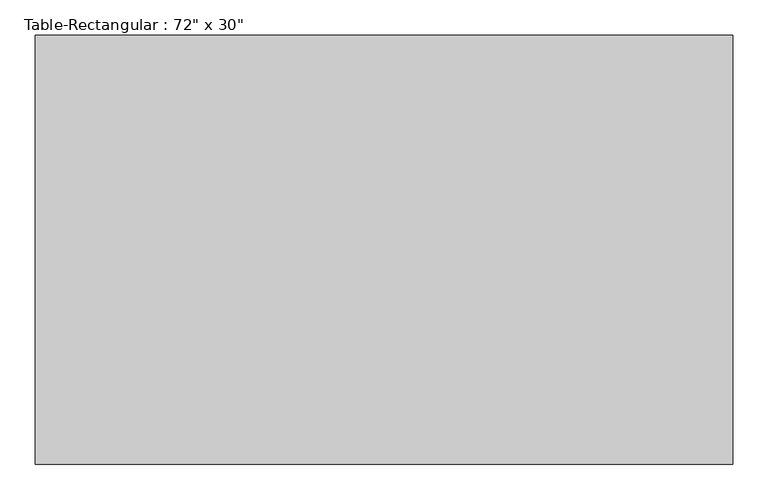
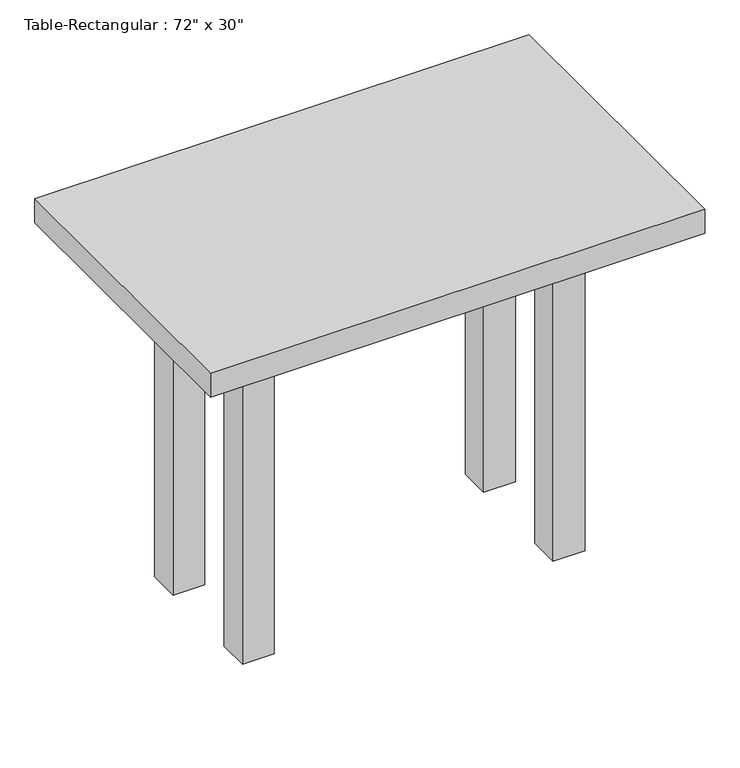
"""IFC4 building model written with IfcOpenShell, lengths in millimetres: furniture geometry."""

from ifc_helpers import new_model, si_unit, frame, origin, origin_with_axes, place, context, project, spatial, polyline, outline, extrude, source, transform, mapped, element, save


def furniture_d861f60e(model_context):
    return source(origin(), model_context, "Body", "SweptSolid", [
        extrude(outline(polyline([(279.4, 114.3), (279.4, 88.9), (-279.4, 88.9), (-279.4, 114.3), (279.4, 114.3)])), frame((0.0, 0.0, 609.6), z_axis=(0.0, 0.0, 1.0), x_axis=(1.0, 0.0, 0.0)), (0.0, 0.0, 1.0), 101.6),
        extrude(outline(polyline([(279.4, -114.3), (-279.4, -114.3), (-279.4, -88.9), (279.4, -88.9), (279.4, -114.3)])), frame((0.0, 0.0, 609.6), z_axis=(0.0, 0.0, 1.0), x_axis=(1.0, 0.0, 0.0)), (0.0, 0.0, 1.0), 101.6),
        extrude(outline(polyline([(-292.1, -88.9), (-317.5, -88.9), (-317.5, 88.9), (-292.1, 88.9), (-292.1, -88.9)])), frame((0.0, 0.0, 609.6), z_axis=(0.0, 0.0, 1.0), x_axis=(1.0, 0.0, 0.0)), (0.0, 0.0, 1.0), 101.6),
        extrude(outline(polyline([(292.1, -88.9), (292.1, 88.9), (317.5, 88.9), (317.5, -88.9), (292.1, -88.9)])), frame((0.0, 0.0, 609.6), z_axis=(0.0, 0.0, 1.0), x_axis=(1.0, 0.0, 0.0)), (0.0, 0.0, 1.0), 101.6),
        extrude(outline(polyline([(495.3, 304.8), (495.3, -304.8), (-495.3, -304.8), (-495.3, 304.8), (495.3, 304.8)])), frame((0.0, 0.0, 711.2), z_axis=(0.0, 0.0, 1.0), x_axis=(1.0, 0.0, 0.0)), (0.0, 0.0, 1.0), 50.8),
        extrude(outline(polyline([(-279.4, 152.4), (-279.4, 88.9), (-342.9, 88.9), (-342.9, 152.4), (-279.4, 152.4)])), origin_with_axes(), (0.0, 0.0, 1.0), 711.2),
        extrude(outline(polyline([(279.4, 152.4), (342.9, 152.4), (342.9, 88.9), (279.4, 88.9), (279.4, 152.4)])), origin_with_axes(), (0.0, 0.0, 1.0), 711.2),
        extrude(outline(polyline([(-279.4, -152.4), (-342.9, -152.4), (-342.9, -88.9), (-279.4, -88.9), (-279.4, -152.4)])), origin_with_axes(), (0.0, 0.0, 1.0), 711.2),
        extrude(outline(polyline([(279.4, -152.4), (279.4, -88.9), (342.9, -88.9), (342.9, -152.4), (279.4, -152.4)])), origin_with_axes(), (0.0, 0.0, 1.0), 711.2),
    ])


if __name__ == "__main__":
    model = new_model("IFC4")
    model_context = context("Model", 3, world=origin())
    ifc_project = project(units=[si_unit("LENGTHUNIT", "METRE", prefix="MILLI")], contexts=[model_context])
    site = spatial("IfcSite", under=ifc_project)
    building = spatial("IfcBuilding", under=site)
    placement = place(None, origin())
    furniture_shape = furniture_d861f60e(model_context)
    element("IfcFurniture", 1, ObjectType="Table-Rectangular : 72\" x 30\"", at=placement, inside=building, context=model_context, shape_type="MappedRepresentation", body=[
        mapped(furniture_shape, transform((0.0, 0.0, 0.0), x_axis=(1.0, 0.0, 0.0), y_axis=(0.0, 1.0, 0.0), z_axis=(0.0, 0.0, 1.0))),
    ])
    save(model, "model.ifc")

# Revit data of these elements
# Type "Table-Rectangular : 72\" x 30\""
#   Assembly Code = "E2020200"
#   Height = 2' - 6"
#   Length = 3' - 3"
#   Width = 2' - 0"
#   Base Material = Birch
#   Top Material = Birch
#   Default Elevation = 0
# Element 1 (IfcFurniture, "Table-Rectangular : 72\" x 30\"")
#   Materials on its faces: "Birch"
# Materials
#   "Birch": class "Wood", colour RGB 224 178 126, transparency 0, Description = "Betula Alleghaniensis", Cost = 0
